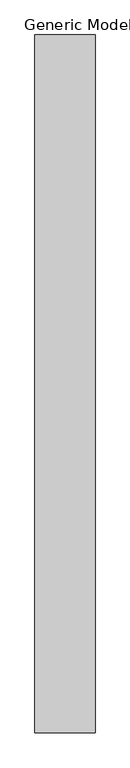
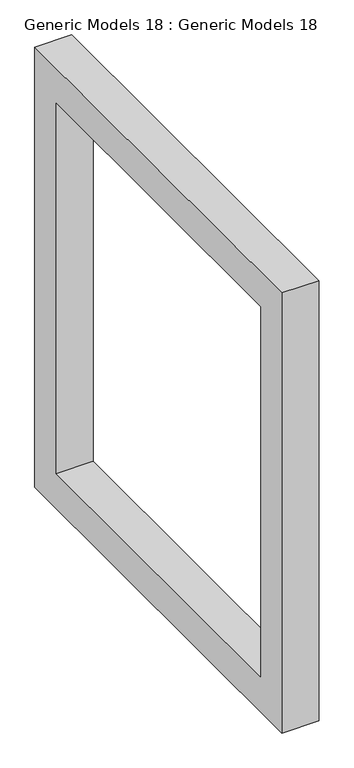
"""IFC4 building model written with IfcOpenShell, lengths in millimetres: proxy geometry, Generic Models 18 : Generic Models 18."""

from ifc_helpers import new_model, si_unit, frame, origin, place, context, project, spatial, polyline, outline, extrude, source, transform, mapped, element, save


def generic_models_18_generic_models_18_2803ece5(model_context):
    return source(origin(), model_context, "Body", "SweptSolid", [
        extrude(outline(polyline([(4881.9172538, 2692.4), (6355.1172538, 2692.4), (6355.1172538, 1092.2), (4881.9172538, 1092.2), (4881.9172538, 2692.4)]), holes=[polyline([(5008.9172538, 2565.4), (5008.9172538, 1219.2), (6228.1172538, 1219.2), (6228.1172538, 2565.4), (5008.9172538, 2565.4)])]), frame((-9825.1482439, 0.0, 0.0), z_axis=(1.0, 0.0, 0.0), x_axis=(0.0, 1.0, 0.0)), (0.0, 0.0, 1.0), 127.0),
    ])


if __name__ == "__main__":
    model = new_model("IFC4")
    model_context = context("Model", 3, world=origin())
    ifc_project = project(units=[si_unit("LENGTHUNIT", "METRE", prefix="MILLI")], contexts=[model_context])
    site = spatial("IfcSite", under=ifc_project)
    building = spatial("IfcBuilding", under=site)
    placement = place(None, origin())
    generic_models_18_generic_models_18_shape = generic_models_18_generic_models_18_2803ece5(model_context)
    element("IfcBuildingElementProxy", 1, Name="Generic Models 18 : Generic Models 18", ObjectType="Generic Models 18 : Generic Models 18", at=placement, inside=building, context=model_context, shape_type="MappedRepresentation", body=[
        mapped(generic_models_18_generic_models_18_shape, transform((0.0, 0.0, 0.0), x_axis=(1.0, 0.0, 0.0), y_axis=(0.0, 1.0, 0.0), z_axis=(0.0, 0.0, 1.0))),
    ])
    save(model, "model.ifc")

# Revit data of these elements
# Element 1 (IfcBuildingElementProxy, "Generic Models 18 : Generic Models 18")
#   Materials on its faces: "BLACK"
# Materials
#   "BLACK": class "Generic", colour RGB 120 120 120, transparency 0, Cost = 0
